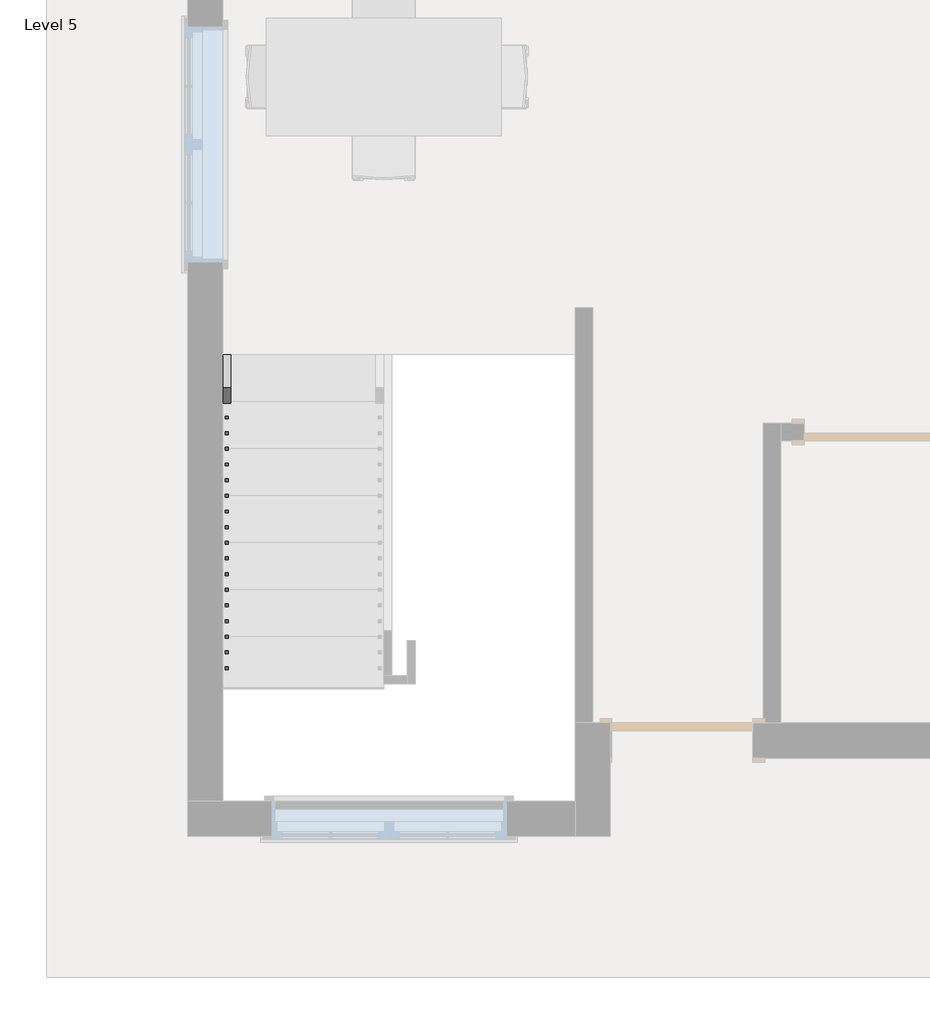
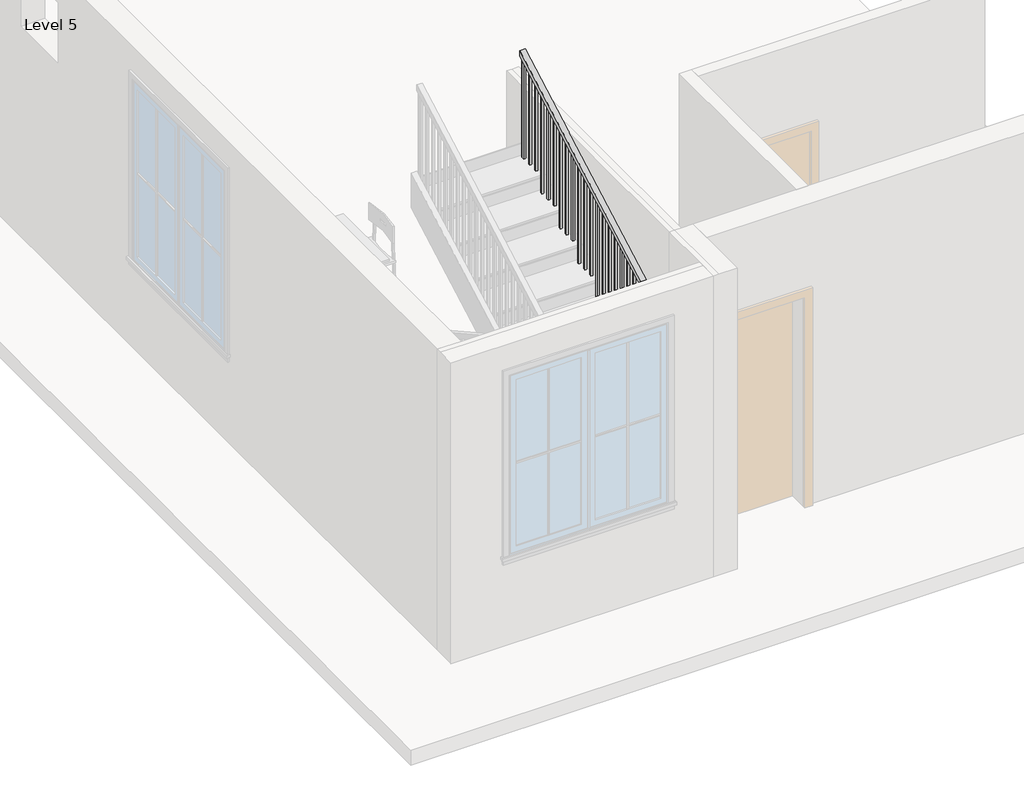
# One storey, part 2 of 3: 1 railing.
"""IFC4 building model written with IfcOpenShell, lengths in millimetres."""

from ifc_helpers import new_model, si_unit, frame, origin, place, context, project, spatial, polyline, outline, extrude, faceted_brep, element, save

model = new_model("IFC4")

# Units and contexts
model_context = context("Model", 3, world=origin())
ifc_project = project(units=[si_unit("LENGTHUNIT", "METRE", prefix="MILLI")], contexts=[model_context])

# Site, building, storey
site = spatial("IfcSite", under=ifc_project)
building = spatial("IfcBuilding", under=site)
storey = spatial("IfcBuildingStorey", under=building, Name="Level 5", Elevation=12649.2)

# Railing
placement = place(None, origin())
element("IfcRailing", 1, ObjectType="Handrail - Rectangular", at=placement, inside=storey, context=model_context, shape_type="SolidModel", body=[
    faceted_brep([(-4181.480864, -3571.6080018, 13732.9333333), (-4181.480864, -3571.6080018, 13674.820221), (-4232.280864, -3571.6080018, 13674.820221), (-4232.280864, -3571.6080018, 13732.9333333), (-4181.480864, -5705.2080018, 14918.2666667), (-4181.480864, -5718.371604, 14867.4666667), (-4232.280864, -5718.371604, 14867.4666667), (-4232.280864, -5705.2080018, 14918.2666667), (-4181.480864, -6416.4080018, 14918.2666667), (-4181.480864, -6416.4080018, 14867.4666667), (-4232.280864, -6467.2080018, 14867.4666667), (-4232.280864, -6467.2080018, 14918.2666667), (-1997.080864, -6416.4080018, 14918.2666667), (-1997.080864, -6416.4080018, 14867.4666667), (-1946.280864, -6467.2080018, 14867.4666667), (-1946.280864, -6467.2080018, 14918.2666667), (-1997.080864, -5705.2080018, 14918.2666667), (-1997.080864, -5692.0443995, 14867.4666667), (-1946.280864, -5692.0443995, 14867.4666667), (-1946.280864, -5705.2080018, 14918.2666667), (-1997.080864, -3571.6080018, 16103.6), (-1946.280864, -3571.6080018, 16103.6), (-1946.280864, -3571.6080018, 16045.4868876), (-1997.080864, -3571.6080018, 16045.4868876)], [[[0, 1, 2, 3]], [[1, 0, 4, 5]], [[2, 1, 5, 6]], [[3, 2, 6, 7]], [[0, 3, 7, 4]], [[5, 4, 8, 9]], [[6, 5, 9, 10]], [[7, 6, 10, 11]], [[4, 7, 11, 8]], [[9, 8, 12, 13]], [[10, 9, 13, 14]], [[11, 10, 14, 15]], [[8, 11, 15, 12]], [[13, 12, 16, 17]], [[14, 13, 17, 18]], [[15, 14, 18, 19]], [[12, 15, 19, 16]], [[20, 21, 22, 23]], [[17, 16, 20, 23]], [[18, 17, 23, 22]], [[19, 18, 22, 21]], [[16, 19, 21, 20]]]),
    extrude(outline(polyline([(-3606.5330018, 16026.0841099), (-3587.4830018, 16036.6674432), (-3587.4830018, 15019.8666667), (-3606.5330018, 15019.8666667), (-3606.5330018, 16026.0841099)])), frame((-1981.205864, 0.0, 0.0), z_axis=(1.0, 0.0, 0.0), x_axis=(0.0, 1.0, 0.0)), (0.0, 0.0, 1.0), 19.05),
    extrude(outline(polyline([(-3708.1330018, 15969.6396654), (-3689.0830018, 15980.2229988), (-3689.0830018, 15019.8666667), (-3708.1330018, 15019.8666667), (-3708.1330018, 15969.6396654)])), frame((-1981.205864, 0.0, 0.0), z_axis=(1.0, 0.0, 0.0), x_axis=(0.0, 1.0, 0.0)), (0.0, 0.0, 1.0), 19.05),
    extrude(outline(polyline([(-3809.7330018, 15913.195221), (-3790.6830018, 15923.7785543), (-3790.6830018, 15019.8666667), (-3809.7330018, 15019.8666667), (-3809.7330018, 15913.195221)])), frame((-1981.205864, 0.0, 0.0), z_axis=(1.0, 0.0, 0.0), x_axis=(0.0, 1.0, 0.0)), (0.0, 0.0, 1.0), 19.05),
    extrude(outline(polyline([(-3911.3330018, 15856.7507765), (-3892.2830018, 15867.3341099), (-3892.2830018, 14850.5333333), (-3911.3330018, 14850.5333333), (-3911.3330018, 15856.7507765)])), frame((-1981.205864, 0.0, 0.0), z_axis=(1.0, 0.0, 0.0), x_axis=(0.0, 1.0, 0.0)), (0.0, 0.0, 1.0), 19.05),
    extrude(outline(polyline([(-4012.9330018, 15800.3063321), (-3993.8830018, 15810.8896654), (-3993.8830018, 14850.5333333), (-4012.9330018, 14850.5333333), (-4012.9330018, 15800.3063321)])), frame((-1981.205864, 0.0, 0.0), z_axis=(1.0, 0.0, 0.0), x_axis=(0.0, 1.0, 0.0)), (0.0, 0.0, 1.0), 19.05),
    extrude(outline(polyline([(-4114.5330018, 15743.8618876), (-4095.4830018, 15754.445221), (-4095.4830018, 14850.5333333), (-4114.5330018, 14850.5333333), (-4114.5330018, 15743.8618876)])), frame((-1981.205864, 0.0, 0.0), z_axis=(1.0, 0.0, 0.0), x_axis=(0.0, 1.0, 0.0)), (0.0, 0.0, 1.0), 19.05),
    extrude(outline(polyline([(-4216.1330018, 15687.4174432), (-4197.0830018, 15698.0007765), (-4197.0830018, 14681.2), (-4216.1330018, 14681.2), (-4216.1330018, 15687.4174432)])), frame((-1981.205864, 0.0, 0.0), z_axis=(1.0, 0.0, 0.0), x_axis=(0.0, 1.0, 0.0)), (0.0, 0.0, 1.0), 19.05),
    extrude(outline(polyline([(-4317.7330018, 15630.9729988), (-4298.6830018, 15641.5563321), (-4298.6830018, 14681.2), (-4317.7330018, 14681.2), (-4317.7330018, 15630.9729988)])), frame((-1981.205864, 0.0, 0.0), z_axis=(1.0, 0.0, 0.0), x_axis=(0.0, 1.0, 0.0)), (0.0, 0.0, 1.0), 19.05),
    extrude(outline(polyline([(-4419.3330018, 15574.5285543), (-4400.2830018, 15585.1118876), (-4400.2830018, 14681.2), (-4419.3330018, 14681.2), (-4419.3330018, 15574.5285543)])), frame((-1981.205864, 0.0, 0.0), z_axis=(1.0, 0.0, 0.0), x_axis=(0.0, 1.0, 0.0)), (0.0, 0.0, 1.0), 19.05),
    extrude(outline(polyline([(-4520.9330018, 15518.0841099), (-4501.8830018, 15528.6674432), (-4501.8830018, 14511.8666667), (-4520.9330018, 14511.8666667), (-4520.9330018, 15518.0841099)])), frame((-1981.205864, 0.0, 0.0), z_axis=(1.0, 0.0, 0.0), x_axis=(0.0, 1.0, 0.0)), (0.0, 0.0, 1.0), 19.05),
    extrude(outline(polyline([(-4622.5330018, 15461.6396654), (-4603.4830018, 15472.2229988), (-4603.4830018, 14511.8666667), (-4622.5330018, 14511.8666667), (-4622.5330018, 15461.6396654)])), frame((-1981.205864, 0.0, 0.0), z_axis=(1.0, 0.0, 0.0), x_axis=(0.0, 1.0, 0.0)), (0.0, 0.0, 1.0), 19.05),
    extrude(outline(polyline([(-4724.1330018, 15405.195221), (-4705.0830018, 15415.7785543), (-4705.0830018, 14511.8666667), (-4724.1330018, 14511.8666667), (-4724.1330018, 15405.195221)])), frame((-1981.205864, 0.0, 0.0), z_axis=(1.0, 0.0, 0.0), x_axis=(0.0, 1.0, 0.0)), (0.0, 0.0, 1.0), 19.05),
    extrude(outline(polyline([(-4825.7330018, 15348.7507765), (-4806.6830018, 15359.3341099), (-4806.6830018, 14342.5333333), (-4825.7330018, 14342.5333333), (-4825.7330018, 15348.7507765)])), frame((-1981.205864, 0.0, 0.0), z_axis=(1.0, 0.0, 0.0), x_axis=(0.0, 1.0, 0.0)), (0.0, 0.0, 1.0), 19.05),
    extrude(outline(polyline([(-4927.3330018, 15292.3063321), (-4908.2830018, 15302.8896654), (-4908.2830018, 14342.5333333), (-4927.3330018, 14342.5333333), (-4927.3330018, 15292.3063321)])), frame((-1981.205864, 0.0, 0.0), z_axis=(1.0, 0.0, 0.0), x_axis=(0.0, 1.0, 0.0)), (0.0, 0.0, 1.0), 19.05),
    extrude(outline(polyline([(-5028.9330018, 15235.8618876), (-5009.8830018, 15246.445221), (-5009.8830018, 14342.5333333), (-5028.9330018, 14342.5333333), (-5028.9330018, 15235.8618876)])), frame((-1981.205864, 0.0, 0.0), z_axis=(1.0, 0.0, 0.0), x_axis=(0.0, 1.0, 0.0)), (0.0, 0.0, 1.0), 19.05),
    extrude(outline(polyline([(-5130.5330018, 15179.4174432), (-5111.4830018, 15190.0007765), (-5111.4830018, 14173.2), (-5130.5330018, 14173.2), (-5130.5330018, 15179.4174432)])), frame((-1981.205864, 0.0, 0.0), z_axis=(1.0, 0.0, 0.0), x_axis=(0.0, 1.0, 0.0)), (0.0, 0.0, 1.0), 19.05),
    extrude(outline(polyline([(-5232.1330018, 15122.9729988), (-5213.0830018, 15133.5563321), (-5213.0830018, 14173.2), (-5232.1330018, 14173.2), (-5232.1330018, 15122.9729988)])), frame((-1981.205864, 0.0, 0.0), z_axis=(1.0, 0.0, 0.0), x_axis=(0.0, 1.0, 0.0)), (0.0, 0.0, 1.0), 19.05),
    extrude(outline(polyline([(-5333.7330018, 15066.5285543), (-5314.6830018, 15077.1118876), (-5314.6830018, 14173.2), (-5333.7330018, 14173.2), (-5333.7330018, 15066.5285543)])), frame((-1981.205864, 0.0, 0.0), z_axis=(1.0, 0.0, 0.0), x_axis=(0.0, 1.0, 0.0)), (0.0, 0.0, 1.0), 19.05),
    extrude(outline(polyline([(-5435.3330018, 15010.0841099), (-5416.2830018, 15020.6674432), (-5416.2830018, 14003.8666667), (-5435.3330018, 14003.8666667), (-5435.3330018, 15010.0841099)])), frame((-1981.205864, 0.0, 0.0), z_axis=(1.0, 0.0, 0.0), x_axis=(0.0, 1.0, 0.0)), (0.0, 0.0, 1.0), 19.05),
    extrude(outline(polyline([(-5536.9330018, 14953.6396654), (-5517.8830018, 14964.2229988), (-5517.8830018, 14003.8666667), (-5536.9330018, 14003.8666667), (-5536.9330018, 14953.6396654)])), frame((-1981.205864, 0.0, 0.0), z_axis=(1.0, 0.0, 0.0), x_axis=(0.0, 1.0, 0.0)), (0.0, 0.0, 1.0), 19.05),
    extrude(outline(polyline([(-5638.5330018, 14897.195221), (-5619.4830018, 14907.7785543), (-5619.4830018, 14003.8666667), (-5638.5330018, 14003.8666667), (-5638.5330018, 14897.195221)])), frame((-1981.205864, 0.0, 0.0), z_axis=(1.0, 0.0, 0.0), x_axis=(0.0, 1.0, 0.0)), (0.0, 0.0, 1.0), 19.05),
    extrude(outline(polyline([(-1962.155864, -5740.1330018), (-1981.205864, -5740.1330018), (-1981.205864, -5721.0830018), (-1962.155864, -5721.0830018), (-1962.155864, -5740.1330018)])), frame((0.0, 0.0, 14003.8666667), z_axis=(0.0, 0.0, 1.0), x_axis=(1.0, 0.0, 0.0)), (0.0, 0.0, 1.0), 863.6),
    extrude(outline(polyline([(-1962.155864, -5841.7330018), (-1981.205864, -5841.7330018), (-1981.205864, -5822.6830018), (-1962.155864, -5822.6830018), (-1962.155864, -5841.7330018)])), frame((0.0, 0.0, 14003.8666667), z_axis=(0.0, 0.0, 1.0), x_axis=(1.0, 0.0, 0.0)), (0.0, 0.0, 1.0), 863.6),
    extrude(outline(polyline([(-1962.155864, -5943.3330018), (-1981.205864, -5943.3330018), (-1981.205864, -5924.2830018), (-1962.155864, -5924.2830018), (-1962.155864, -5943.3330018)])), frame((0.0, 0.0, 14003.8666667), z_axis=(0.0, 0.0, 1.0), x_axis=(1.0, 0.0, 0.0)), (0.0, 0.0, 1.0), 863.6),
    extrude(outline(polyline([(-1962.155864, -6044.9330018), (-1981.205864, -6044.9330018), (-1981.205864, -6025.8830018), (-1962.155864, -6025.8830018), (-1962.155864, -6044.9330018)])), frame((0.0, 0.0, 14003.8666667), z_axis=(0.0, 0.0, 1.0), x_axis=(1.0, 0.0, 0.0)), (0.0, 0.0, 1.0), 863.6),
    extrude(outline(polyline([(-1962.155864, -6146.5330018), (-1981.205864, -6146.5330018), (-1981.205864, -6127.4830018), (-1962.155864, -6127.4830018), (-1962.155864, -6146.5330018)])), frame((0.0, 0.0, 14003.8666667), z_axis=(0.0, 0.0, 1.0), x_axis=(1.0, 0.0, 0.0)), (0.0, 0.0, 1.0), 863.6),
    extrude(outline(polyline([(-1962.155864, -6248.1330018), (-1981.205864, -6248.1330018), (-1981.205864, -6229.0830018), (-1962.155864, -6229.0830018), (-1962.155864, -6248.1330018)])), frame((0.0, 0.0, 14003.8666667), z_axis=(0.0, 0.0, 1.0), x_axis=(1.0, 0.0, 0.0)), (0.0, 0.0, 1.0), 863.6),
    extrude(outline(polyline([(-1962.155864, -6349.7330018), (-1981.205864, -6349.7330018), (-1981.205864, -6330.6830018), (-1962.155864, -6330.6830018), (-1962.155864, -6349.7330018)])), frame((0.0, 0.0, 14003.8666667), z_axis=(0.0, 0.0, 1.0), x_axis=(1.0, 0.0, 0.0)), (0.0, 0.0, 1.0), 863.6),
    extrude(outline(polyline([(-2082.805864, -6451.3330018), (-2082.805864, -6432.2830018), (-2063.755864, -6432.2830018), (-2063.755864, -6451.3330018), (-2082.805864, -6451.3330018)])), frame((0.0, 0.0, 14003.8666667), z_axis=(0.0, 0.0, 1.0), x_axis=(1.0, 0.0, 0.0)), (0.0, 0.0, 1.0), 863.6),
    extrude(outline(polyline([(-2184.405864, -6451.3330018), (-2184.405864, -6432.2830018), (-2165.355864, -6432.2830018), (-2165.355864, -6451.3330018), (-2184.405864, -6451.3330018)])), frame((0.0, 0.0, 14003.8666667), z_axis=(0.0, 0.0, 1.0), x_axis=(1.0, 0.0, 0.0)), (0.0, 0.0, 1.0), 863.6),
    extrude(outline(polyline([(-2286.005864, -6451.3330018), (-2286.005864, -6432.2830018), (-2266.955864, -6432.2830018), (-2266.955864, -6451.3330018), (-2286.005864, -6451.3330018)])), frame((0.0, 0.0, 14003.8666667), z_axis=(0.0, 0.0, 1.0), x_axis=(1.0, 0.0, 0.0)), (0.0, 0.0, 1.0), 863.6),
    extrude(outline(polyline([(-2387.605864, -6451.3330018), (-2387.605864, -6432.2830018), (-2368.555864, -6432.2830018), (-2368.555864, -6451.3330018), (-2387.605864, -6451.3330018)])), frame((0.0, 0.0, 14003.8666667), z_axis=(0.0, 0.0, 1.0), x_axis=(1.0, 0.0, 0.0)), (0.0, 0.0, 1.0), 863.6),
    extrude(outline(polyline([(-2489.205864, -6451.3330018), (-2489.205864, -6432.2830018), (-2470.155864, -6432.2830018), (-2470.155864, -6451.3330018), (-2489.205864, -6451.3330018)])), frame((0.0, 0.0, 14003.8666667), z_axis=(0.0, 0.0, 1.0), x_axis=(1.0, 0.0, 0.0)), (0.0, 0.0, 1.0), 863.6),
    extrude(outline(polyline([(-2590.805864, -6451.3330018), (-2590.805864, -6432.2830018), (-2571.755864, -6432.2830018), (-2571.755864, -6451.3330018), (-2590.805864, -6451.3330018)])), frame((0.0, 0.0, 14003.8666667), z_axis=(0.0, 0.0, 1.0), x_axis=(1.0, 0.0, 0.0)), (0.0, 0.0, 1.0), 863.6),
    extrude(outline(polyline([(-2692.405864, -6451.3330018), (-2692.405864, -6432.2830018), (-2673.355864, -6432.2830018), (-2673.355864, -6451.3330018), (-2692.405864, -6451.3330018)])), frame((0.0, 0.0, 14003.8666667), z_axis=(0.0, 0.0, 1.0), x_axis=(1.0, 0.0, 0.0)), (0.0, 0.0, 1.0), 863.6),
    extrude(outline(polyline([(-2794.005864, -6451.3330018), (-2794.005864, -6432.2830018), (-2774.955864, -6432.2830018), (-2774.955864, -6451.3330018), (-2794.005864, -6451.3330018)])), frame((0.0, 0.0, 14003.8666667), z_axis=(0.0, 0.0, 1.0), x_axis=(1.0, 0.0, 0.0)), (0.0, 0.0, 1.0), 863.6),
    extrude(outline(polyline([(-2895.605864, -6451.3330018), (-2895.605864, -6432.2830018), (-2876.555864, -6432.2830018), (-2876.555864, -6451.3330018), (-2895.605864, -6451.3330018)])), frame((0.0, 0.0, 14003.8666667), z_axis=(0.0, 0.0, 1.0), x_axis=(1.0, 0.0, 0.0)), (0.0, 0.0, 1.0), 863.6),
    extrude(outline(polyline([(-2997.205864, -6451.3330018), (-2997.205864, -6432.2830018), (-2978.155864, -6432.2830018), (-2978.155864, -6451.3330018), (-2997.205864, -6451.3330018)])), frame((0.0, 0.0, 14003.8666667), z_axis=(0.0, 0.0, 1.0), x_axis=(1.0, 0.0, 0.0)), (0.0, 0.0, 1.0), 863.6),
    extrude(outline(polyline([(-3098.805864, -6451.3330018), (-3098.805864, -6432.2830018), (-3079.755864, -6432.2830018), (-3079.755864, -6451.3330018), (-3098.805864, -6451.3330018)])), frame((0.0, 0.0, 14003.8666667), z_axis=(0.0, 0.0, 1.0), x_axis=(1.0, 0.0, 0.0)), (0.0, 0.0, 1.0), 863.6),
    extrude(outline(polyline([(-3200.405864, -6451.3330018), (-3200.405864, -6432.2830018), (-3181.355864, -6432.2830018), (-3181.355864, -6451.3330018), (-3200.405864, -6451.3330018)])), frame((0.0, 0.0, 14003.8666667), z_axis=(0.0, 0.0, 1.0), x_axis=(1.0, 0.0, 0.0)), (0.0, 0.0, 1.0), 863.6),
    extrude(outline(polyline([(-3302.005864, -6451.3330018), (-3302.005864, -6432.2830018), (-3282.955864, -6432.2830018), (-3282.955864, -6451.3330018), (-3302.005864, -6451.3330018)])), frame((0.0, 0.0, 14003.8666667), z_axis=(0.0, 0.0, 1.0), x_axis=(1.0, 0.0, 0.0)), (0.0, 0.0, 1.0), 863.6),
    extrude(outline(polyline([(-3403.605864, -6451.3330018), (-3403.605864, -6432.2830018), (-3384.555864, -6432.2830018), (-3384.555864, -6451.3330018), (-3403.605864, -6451.3330018)])), frame((0.0, 0.0, 14003.8666667), z_axis=(0.0, 0.0, 1.0), x_axis=(1.0, 0.0, 0.0)), (0.0, 0.0, 1.0), 863.6),
    extrude(outline(polyline([(-3505.205864, -6451.3330018), (-3505.205864, -6432.2830018), (-3486.155864, -6432.2830018), (-3486.155864, -6451.3330018), (-3505.205864, -6451.3330018)])), frame((0.0, 0.0, 14003.8666667), z_axis=(0.0, 0.0, 1.0), x_axis=(1.0, 0.0, 0.0)), (0.0, 0.0, 1.0), 863.6),
    extrude(outline(polyline([(-3606.805864, -6451.3330018), (-3606.805864, -6432.2830018), (-3587.755864, -6432.2830018), (-3587.755864, -6451.3330018), (-3606.805864, -6451.3330018)])), frame((0.0, 0.0, 14003.8666667), z_axis=(0.0, 0.0, 1.0), x_axis=(1.0, 0.0, 0.0)), (0.0, 0.0, 1.0), 863.6),
    extrude(outline(polyline([(-3708.405864, -6451.3330018), (-3708.405864, -6432.2830018), (-3689.355864, -6432.2830018), (-3689.355864, -6451.3330018), (-3708.405864, -6451.3330018)])), frame((0.0, 0.0, 14003.8666667), z_axis=(0.0, 0.0, 1.0), x_axis=(1.0, 0.0, 0.0)), (0.0, 0.0, 1.0), 863.6),
    extrude(outline(polyline([(-3810.005864, -6451.3330018), (-3810.005864, -6432.2830018), (-3790.955864, -6432.2830018), (-3790.955864, -6451.3330018), (-3810.005864, -6451.3330018)])), frame((0.0, 0.0, 14003.8666667), z_axis=(0.0, 0.0, 1.0), x_axis=(1.0, 0.0, 0.0)), (0.0, 0.0, 1.0), 863.6),
    extrude(outline(polyline([(-3911.605864, -6451.3330018), (-3911.605864, -6432.2830018), (-3892.555864, -6432.2830018), (-3892.555864, -6451.3330018), (-3911.605864, -6451.3330018)])), frame((0.0, 0.0, 14003.8666667), z_axis=(0.0, 0.0, 1.0), x_axis=(1.0, 0.0, 0.0)), (0.0, 0.0, 1.0), 863.6),
    extrude(outline(polyline([(-4013.205864, -6451.3330018), (-4013.205864, -6432.2830018), (-3994.155864, -6432.2830018), (-3994.155864, -6451.3330018), (-4013.205864, -6451.3330018)])), frame((0.0, 0.0, 14003.8666667), z_axis=(0.0, 0.0, 1.0), x_axis=(1.0, 0.0, 0.0)), (0.0, 0.0, 1.0), 863.6),
    extrude(outline(polyline([(-4114.805864, -6451.3330018), (-4114.805864, -6432.2830018), (-4095.755864, -6432.2830018), (-4095.755864, -6451.3330018), (-4114.805864, -6451.3330018)])), frame((0.0, 0.0, 14003.8666667), z_axis=(0.0, 0.0, 1.0), x_axis=(1.0, 0.0, 0.0)), (0.0, 0.0, 1.0), 863.6),
    extrude(outline(polyline([(-4216.405864, -6406.8830018), (-4197.355864, -6406.8830018), (-4197.355864, -6425.9330018), (-4216.405864, -6425.9330018), (-4216.405864, -6406.8830018)])), frame((0.0, 0.0, 14003.8666667), z_axis=(0.0, 0.0, 1.0), x_axis=(1.0, 0.0, 0.0)), (0.0, 0.0, 1.0), 863.6),
    extrude(outline(polyline([(-4216.405864, -6305.2830018), (-4197.355864, -6305.2830018), (-4197.355864, -6324.3330018), (-4216.405864, -6324.3330018), (-4216.405864, -6305.2830018)])), frame((0.0, 0.0, 14003.8666667), z_axis=(0.0, 0.0, 1.0), x_axis=(1.0, 0.0, 0.0)), (0.0, 0.0, 1.0), 863.6),
    extrude(outline(polyline([(-4216.405864, -6203.6830018), (-4197.355864, -6203.6830018), (-4197.355864, -6222.7330018), (-4216.405864, -6222.7330018), (-4216.405864, -6203.6830018)])), frame((0.0, 0.0, 14003.8666667), z_axis=(0.0, 0.0, 1.0), x_axis=(1.0, 0.0, 0.0)), (0.0, 0.0, 1.0), 863.6),
    extrude(outline(polyline([(-4216.405864, -6102.0830018), (-4197.355864, -6102.0830018), (-4197.355864, -6121.1330018), (-4216.405864, -6121.1330018), (-4216.405864, -6102.0830018)])), frame((0.0, 0.0, 14003.8666667), z_axis=(0.0, 0.0, 1.0), x_axis=(1.0, 0.0, 0.0)), (0.0, 0.0, 1.0), 863.6),
    extrude(outline(polyline([(-4216.405864, -6000.4830018), (-4197.355864, -6000.4830018), (-4197.355864, -6019.5330018), (-4216.405864, -6019.5330018), (-4216.405864, -6000.4830018)])), frame((0.0, 0.0, 14003.8666667), z_axis=(0.0, 0.0, 1.0), x_axis=(1.0, 0.0, 0.0)), (0.0, 0.0, 1.0), 863.6),
    extrude(outline(polyline([(-4216.405864, -5898.8830018), (-4197.355864, -5898.8830018), (-4197.355864, -5917.9330018), (-4216.405864, -5917.9330018), (-4216.405864, -5898.8830018)])), frame((0.0, 0.0, 14003.8666667), z_axis=(0.0, 0.0, 1.0), x_axis=(1.0, 0.0, 0.0)), (0.0, 0.0, 1.0), 863.6),
    extrude(outline(polyline([(-4216.405864, -5797.2830018), (-4197.355864, -5797.2830018), (-4197.355864, -5816.3330018), (-4216.405864, -5816.3330018), (-4216.405864, -5797.2830018)])), frame((0.0, 0.0, 14003.8666667), z_axis=(0.0, 0.0, 1.0), x_axis=(1.0, 0.0, 0.0)), (0.0, 0.0, 1.0), 863.6),
    extrude(outline(polyline([(-5714.7330018, 14865.445221), (-5695.6830018, 14854.8618876), (-5695.6830018, 14003.8666667), (-5714.7330018, 14003.8666667), (-5714.7330018, 14865.445221)])), frame((-4216.405864, 0.0, 0.0), z_axis=(1.0, 0.0, 0.0), x_axis=(0.0, 1.0, 0.0)), (0.0, 0.0, 1.0), 19.05),
    extrude(outline(polyline([(-5613.1330018, 14809.0007765), (-5594.0830018, 14798.4174432), (-5594.0830018, 13834.5333333), (-5613.1330018, 13834.5333333), (-5613.1330018, 14809.0007765)])), frame((-4216.405864, 0.0, 0.0), z_axis=(1.0, 0.0, 0.0), x_axis=(0.0, 1.0, 0.0)), (0.0, 0.0, 1.0), 19.05),
    extrude(outline(polyline([(-5511.5330018, 14752.5563321), (-5492.4830018, 14741.9729988), (-5492.4830018, 13834.5333333), (-5511.5330018, 13834.5333333), (-5511.5330018, 14752.5563321)])), frame((-4216.405864, 0.0, 0.0), z_axis=(1.0, 0.0, 0.0), x_axis=(0.0, 1.0, 0.0)), (0.0, 0.0, 1.0), 19.05),
    extrude(outline(polyline([(-5409.9330018, 14696.1118876), (-5390.8830018, 14685.5285543), (-5390.8830018, 13834.5333333), (-5409.9330018, 13834.5333333), (-5409.9330018, 14696.1118876)])), frame((-4216.405864, 0.0, 0.0), z_axis=(1.0, 0.0, 0.0), x_axis=(0.0, 1.0, 0.0)), (0.0, 0.0, 1.0), 19.05),
    extrude(outline(polyline([(-5308.3330018, 14639.6674432), (-5289.2830018, 14629.0841099), (-5289.2830018, 13665.2), (-5308.3330018, 13665.2), (-5308.3330018, 14639.6674432)])), frame((-4216.405864, 0.0, 0.0), z_axis=(1.0, 0.0, 0.0), x_axis=(0.0, 1.0, 0.0)), (0.0, 0.0, 1.0), 19.05),
    extrude(outline(polyline([(-5206.7330018, 14583.2229988), (-5187.6830018, 14572.6396654), (-5187.6830018, 13665.2), (-5206.7330018, 13665.2), (-5206.7330018, 14583.2229988)])), frame((-4216.405864, 0.0, 0.0), z_axis=(1.0, 0.0, 0.0), x_axis=(0.0, 1.0, 0.0)), (0.0, 0.0, 1.0), 19.05),
    extrude(outline(polyline([(-5105.1330018, 14526.7785543), (-5086.0830018, 14516.195221), (-5086.0830018, 13665.2), (-5105.1330018, 13665.2), (-5105.1330018, 14526.7785543)])), frame((-4216.405864, 0.0, 0.0), z_axis=(1.0, 0.0, 0.0), x_axis=(0.0, 1.0, 0.0)), (0.0, 0.0, 1.0), 19.05),
    extrude(outline(polyline([(-5003.5330018, 14470.3341099), (-4984.4830018, 14459.7507765), (-4984.4830018, 13495.8666667), (-5003.5330018, 13495.8666667), (-5003.5330018, 14470.3341099)])), frame((-4216.405864, 0.0, 0.0), z_axis=(1.0, 0.0, 0.0), x_axis=(0.0, 1.0, 0.0)), (0.0, 0.0, 1.0), 19.05),
    extrude(outline(polyline([(-4901.9330018, 14413.8896654), (-4882.8830018, 14403.3063321), (-4882.8830018, 13495.8666667), (-4901.9330018, 13495.8666667), (-4901.9330018, 14413.8896654)])), frame((-4216.405864, 0.0, 0.0), z_axis=(1.0, 0.0, 0.0), x_axis=(0.0, 1.0, 0.0)), (0.0, 0.0, 1.0), 19.05),
    extrude(outline(polyline([(-4800.3330018, 14357.445221), (-4781.2830018, 14346.8618876), (-4781.2830018, 13495.8666667), (-4800.3330018, 13495.8666667), (-4800.3330018, 14357.445221)])), frame((-4216.405864, 0.0, 0.0), z_axis=(1.0, 0.0, 0.0), x_axis=(0.0, 1.0, 0.0)), (0.0, 0.0, 1.0), 19.05),
    extrude(outline(polyline([(-4698.7330018, 14301.0007765), (-4679.6830018, 14290.4174432), (-4679.6830018, 13326.5333333), (-4698.7330018, 13326.5333333), (-4698.7330018, 14301.0007765)])), frame((-4216.405864, 0.0, 0.0), z_axis=(1.0, 0.0, 0.0), x_axis=(0.0, 1.0, 0.0)), (0.0, 0.0, 1.0), 19.05),
    extrude(outline(polyline([(-4597.1330018, 14244.5563321), (-4578.0830018, 14233.9729988), (-4578.0830018, 13326.5333333), (-4597.1330018, 13326.5333333), (-4597.1330018, 14244.5563321)])), frame((-4216.405864, 0.0, 0.0), z_axis=(1.0, 0.0, 0.0), x_axis=(0.0, 1.0, 0.0)), (0.0, 0.0, 1.0), 19.05),
    extrude(outline(polyline([(-4495.5330018, 14188.1118876), (-4476.4830018, 14177.5285543), (-4476.4830018, 13326.5333333), (-4495.5330018, 13326.5333333), (-4495.5330018, 14188.1118876)])), frame((-4216.405864, 0.0, 0.0), z_axis=(1.0, 0.0, 0.0), x_axis=(0.0, 1.0, 0.0)), (0.0, 0.0, 1.0), 19.05),
    extrude(outline(polyline([(-4393.9330018, 14131.6674432), (-4374.8830018, 14121.0841099), (-4374.8830018, 13157.2), (-4393.9330018, 13157.2), (-4393.9330018, 14131.6674432)])), frame((-4216.405864, 0.0, 0.0), z_axis=(1.0, 0.0, 0.0), x_axis=(0.0, 1.0, 0.0)), (0.0, 0.0, 1.0), 19.05),
    extrude(outline(polyline([(-4292.3330018, 14075.2229988), (-4273.2830018, 14064.6396654), (-4273.2830018, 13157.2), (-4292.3330018, 13157.2), (-4292.3330018, 14075.2229988)])), frame((-4216.405864, 0.0, 0.0), z_axis=(1.0, 0.0, 0.0), x_axis=(0.0, 1.0, 0.0)), (0.0, 0.0, 1.0), 19.05),
    extrude(outline(polyline([(-4190.7330018, 14018.7785543), (-4171.6830018, 14008.195221), (-4171.6830018, 13157.2), (-4190.7330018, 13157.2), (-4190.7330018, 14018.7785543)])), frame((-4216.405864, 0.0, 0.0), z_axis=(1.0, 0.0, 0.0), x_axis=(0.0, 1.0, 0.0)), (0.0, 0.0, 1.0), 19.05),
    extrude(outline(polyline([(-4089.1330018, 13962.3341099), (-4070.0830018, 13951.7507765), (-4070.0830018, 12987.8666667), (-4089.1330018, 12987.8666667), (-4089.1330018, 13962.3341099)])), frame((-4216.405864, 0.0, 0.0), z_axis=(1.0, 0.0, 0.0), x_axis=(0.0, 1.0, 0.0)), (0.0, 0.0, 1.0), 19.05),
    extrude(outline(polyline([(-3987.5330018, 13905.8896654), (-3968.4830018, 13895.3063321), (-3968.4830018, 12987.8666667), (-3987.5330018, 12987.8666667), (-3987.5330018, 13905.8896654)])), frame((-4216.405864, 0.0, 0.0), z_axis=(1.0, 0.0, 0.0), x_axis=(0.0, 1.0, 0.0)), (0.0, 0.0, 1.0), 19.05),
    extrude(outline(polyline([(-3885.9330018, 13849.445221), (-3866.8830018, 13838.8618876), (-3866.8830018, 12987.8666667), (-3885.9330018, 12987.8666667), (-3885.9330018, 13849.445221)])), frame((-4216.405864, 0.0, 0.0), z_axis=(1.0, 0.0, 0.0), x_axis=(0.0, 1.0, 0.0)), (0.0, 0.0, 1.0), 19.05),
    extrude(outline(polyline([(-3784.3330018, 13793.0007765), (-3765.2830018, 13782.4174432), (-3765.2830018, 12818.5333333), (-3784.3330018, 12818.5333333), (-3784.3330018, 13793.0007765)])), frame((-4216.405864, 0.0, 0.0), z_axis=(1.0, 0.0, 0.0), x_axis=(0.0, 1.0, 0.0)), (0.0, 0.0, 1.0), 19.05),
    extrude(outline(polyline([(-3682.7330018, 13736.5563321), (-3663.6830018, 13725.9729988), (-3663.6830018, 12818.5333333), (-3682.7330018, 12818.5333333), (-3682.7330018, 13736.5563321)])), frame((-4216.405864, 0.0, 0.0), z_axis=(1.0, 0.0, 0.0), x_axis=(0.0, 1.0, 0.0)), (0.0, 0.0, 1.0), 19.05),
    extrude(outline(polyline([(-1981.205864, -6451.3330018), (-1981.205864, -6432.2830018), (-1962.155864, -6432.2830018), (-1962.155864, -6451.3330018), (-1981.205864, -6451.3330018)])), frame((0.0, 0.0, 14003.8666667), z_axis=(0.0, 0.0, 1.0), x_axis=(1.0, 0.0, 0.0)), (0.0, 0.0, 1.0), 863.6),
    extrude(outline(polyline([(-4216.405864, -6432.2830018), (-4197.355864, -6432.2830018), (-4197.355864, -6451.3330018), (-4216.405864, -6451.3330018), (-4216.405864, -6432.2830018)])), frame((0.0, 0.0, 14003.8666667), z_axis=(0.0, 0.0, 1.0), x_axis=(1.0, 0.0, 0.0)), (0.0, 0.0, 1.0), 863.6),
    extrude(outline(polyline([(-3590.6580018, 16034.9035543), (-3571.6080018, 16045.4868876), (-3571.6080018, 15019.8666667), (-3590.6580018, 15019.8666667), (-3590.6580018, 16034.9035543)])), frame((-1981.205864, 0.0, 0.0), z_axis=(1.0, 0.0, 0.0), x_axis=(0.0, 1.0, 0.0)), (0.0, 0.0, 1.0), 19.05),
    extrude(outline(polyline([(-3590.6580018, 13685.4035543), (-3571.6080018, 13674.820221), (-3571.6080018, 12818.5333333), (-3590.6580018, 12818.5333333), (-3590.6580018, 13685.4035543)])), frame((-4216.405864, 0.0, 0.0), z_axis=(1.0, 0.0, 0.0), x_axis=(0.0, 1.0, 0.0)), (0.0, 0.0, 1.0), 19.05),
])

save(model, "model.ifc")

# Revit data of these elements
# Type "Handrail - Rectangular"
#   Assembly Code = "C2010400"
#   built-in parameter 1008612 = 0.0416667 (stored number, unit not read)
#   built-in parameter 1008611 = 0.0416667 (stored number, unit not read)
#   built-in parameter 1008609 = 0.333333 (stored number, unit not read)
#   built-in parameter 1008604 = 0.166667 (stored number, unit not read)
#   built-in parameter 1008603 = 0.166667 (stored number, unit not read)
#   Railing Height = 3' - 0"
#   built-in parameter 1008630 = 2
#   built-in parameter 1008610 = 2
#   built-in parameter 1008618 = Baluster - Square : 3/4"
# Element 1 (IfcRailing, "Handrail - Rectangular")
#   Phase Created = New Construction
